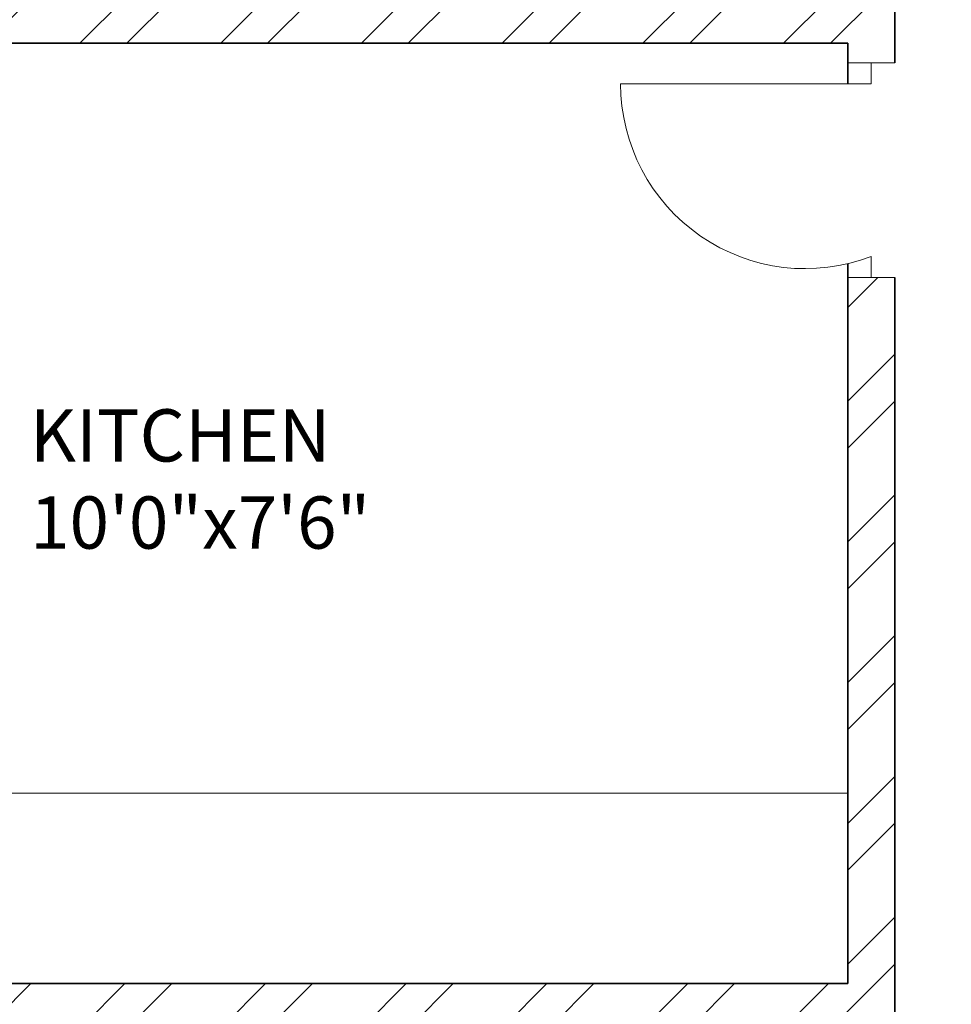
# Model space of a CAD drawing. Units: inches. Extents: x 1885 to 2748, y 783 to 2421.
# Tile 79 of 117: x 2038 to 2127, y 2073 to 2167. Entities that reach past the tile are written whole.
import ezdxf

# ---------------------------------------------------------------- set-up
doc = ezdxf.new("R2010")
doc.units = ezdxf.units.IN
for name, color, linetype, lineweight in [('A-AREA-IDEN', 7, 'Continuous', 18), ('A-DOOR', 31, 'Continuous', 18), ('A-FLOR-CASE', 9, 'Continuous', 18), ('A-WALL', 7, 'Continuous', 35)]:
    doc.layers.add(name, color=color, linetype=linetype, lineweight=lineweight)
doc.layers.add('A-WALL-PATT', color=85, linetype='Continuous', lineweight=13, true_color=0x58ba48)
doc.styles.get("Standard").update_dxf_attribs({"font": 'arial.ttf'})

msp = doc.modelspace()

# ---------------------------------------------------------------- hatches: boundary and pattern name
at = {"layer": 'A-WALL-PATT'}
h = msp.add_hatch(dxfattribs=at)
h.set_pattern_fill('ANSI32', color=256)
h.paths.add_polyline_path([(2007.772, 2318.006), (1980.774, 2318.006), (1980.774, 2281.215), (1985.274, 2281.215), (1985.274, 2313.506), (2007.772, 2313.506), (2007.772, 2315.756)])
h.paths.add_polyline_path([(2094.324, 2318.006), (2067.772, 2318.006), (2067.772, 2313.506), (2094.324, 2313.506), (2094.324, 2315.756)])
h.paths.add_polyline_path([(2131.367, 2315.756), (2131.367, 2318.006), (2131.189, 2318.006), (2112.609, 2318.006), (2112.609, 2313.506), (2117.274, 2313.506), (2117.274, 2255.201), (2121.774, 2255.201), (2121.774, 2313.506), (2131.367, 2313.506)])
h.paths.add_polyline_path([(2190.512, 2318.006), (2155.367, 2318.006), (2155.367, 2313.506), (2169.774, 2313.506), (2169.774, 2229.506), (2121.774, 2229.506), (2121.774, 2233.451), (2119.524, 2233.451), (2117.274, 2233.451), (2117.274, 2201.101), (2121.774, 2201.101), (2121.774, 2225.006), (2169.774, 2225.006), (2169.774, 2165.006), (2306.274, 2165.006), (2306.274, 2066.006), (2310.774, 2066.006), (2344.274, 2066.006), (2486.274, 2066.006), (2486.274, 1886.006), (2483.02, 1886.006), (2483.02, 1881.506), (2486.274, 1881.506), (2486.274, 1880.678), (2490.774, 1880.678), (2490.774, 2070.506), (2344.274, 2070.506), (2310.774, 2070.506), (2310.774, 2165.006), (2310.774, 2173.636), (2308.524, 2173.636), (2306.274, 2173.636), (2306.274, 2169.506), (2174.274, 2169.506), (2174.274, 2313.506), (2190.512, 2313.506), (2190.512, 2315.756)])
h.paths.add_polyline_path([(1985.274, 2221.215), (1980.774, 2221.215), (1980.774, 2165.006), (1992.774, 2165.006), (1992.774, 2141.927), (1997.274, 2141.927), (1997.274, 2165.006), (2117.274, 2165.006), (2117.274, 2163.126), (2121.774, 2163.126), (2121.774, 2172.734), (2119.524, 2172.734), (2117.274, 2172.734), (2117.274, 2169.506), (1985.274, 2169.506)])
h.paths.add_polyline_path([(1997.274, 2105.927), (1992.774, 2105.927), (1992.774, 2070.506), (2016.774, 2070.506), (2016.774, 2059.123), (2019.024, 2059.123), (2021.274, 2059.123), (2021.274, 2070.506), (2117.274, 2070.506), (2117.274, 2022.506), (2114.423, 2022.506), (2114.423, 2018.006), (2123.627, 2018.006), (2123.627, 2020.256), (2123.627, 2022.506), (2121.774, 2022.506), (2121.774, 2142.587), (2119.524, 2142.587), (2117.274, 2142.587), (2117.274, 2075.006), (1997.274, 2075.006)])
h.paths.add_polyline_path([(2092.029, 2020.256), (2092.029, 2022.506), (2021.274, 2022.506), (2021.274, 2035.123), (2016.774, 2035.123), (2016.774, 2018.006), (2016.774, 1978.784), (2021.274, 1978.784), (2021.274, 2018.006), (2092.029, 2018.006)])
h.paths.add_polyline_path([(2260.938, 2022.506), (2153.105, 2022.506), (2153.105, 2020.256), (2153.105, 2018.006), (2155.274, 2018.006), (2155.274, 1886.006), (2107.629, 1886.006), (2107.629, 1881.506), (2182.911, 1881.506), (2182.911, 1883.756), (2182.911, 1886.006), (2159.774, 1886.006), (2159.774, 2018.006), (2260.938, 2018.006), (2260.938, 2020.256)])
h.paths.add_polyline_path([(2047.629, 1883.756), (2047.629, 1886.006), (2021.274, 1886.006), (2021.274, 1918.784), (2019.024, 1918.784), (2016.774, 1918.784), (2016.774, 1881.506), (2047.629, 1881.506)])
h.paths.add_polyline_path([(2306.361, 1883.756), (2306.361, 1886.006), (2296.274, 1886.006), (2296.274, 1982.006), (2316.535, 1982.006), (2316.535, 1984.256), (2316.535, 1986.506), (2296.274, 1986.506), (2296.274, 2022.506), (2289.276, 2022.506), (2289.276, 2018.006), (2291.774, 2018.006), (2291.774, 1886.006), (2242.911, 1886.006), (2242.911, 1881.506), (2306.361, 1881.506)], flags=17)
h.paths.add_polyline_path([(1985.274, 1843.006), (2021.6, 1843.006), (2021.534, 1845.441), (2021.477, 1847.506), (1980.774, 1847.506), (1980.774, 1809.446), (1985.274, 1809.446)])
h.paths.add_polyline_path([(2131.482, 1845.256), (2131.482, 1847.506), (2081.534, 1847.506), (2081.534, 1843.006), (2117.274, 1843.006), (2117.274, 1784.147), (2119.524, 1784.147), (2121.774, 1784.147), (2121.774, 1843.006), (2131.482, 1843.006)])
h.paths.add_polyline_path([(2203.886, 1847.506), (2155.482, 1847.506), (2155.482, 1843.006), (2169.774, 1843.006), (2169.774, 1759.006), (2121.774, 1759.006), (2121.774, 1761.457), (2117.274, 1761.457), (2117.274, 1730.429), (2121.774, 1730.429), (2121.774, 1754.506), (2177.421, 1754.506), (2177.421, 1756.756), (2177.421, 1759.006), (2174.274, 1759.006), (2174.274, 1843.006), (2203.886, 1843.006)])
h.paths.add_polyline_path([(2335.554, 1845.256), (2335.554, 1847.506), (2239.886, 1847.506), (2239.886, 1843.006), (2306.274, 1843.006), (2306.274, 1759.006), (2199.486, 1759.006), (2199.486, 1754.506), (2310.774, 1754.506), (2310.774, 1843.006), (2335.554, 1843.006)])
h.paths.add_polyline_path([(2348.774, 2022.506), (2344.274, 2022.506), (2344.274, 1986.506), (2341.681, 1986.506), (2341.681, 1982.006), (2344.274, 1982.006), (2344.274, 1886.006), (2330.361, 1886.006), (2330.361, 1881.506), (2361.627, 1881.506), (2361.627, 1883.756), (2361.627, 1886.006), (2348.774, 1886.006)], flags=17)
h.paths.add_polyline_path([(2283.251, 2315.756), (2283.251, 2318.006), (2238.512, 2318.006), (2238.512, 2313.506), (2283.251, 2313.506)], flags=17)
h.paths.add_polyline_path([(2363.274, 2348.006), (2388.677, 2348.006), (2388.677, 2350.256), (2388.677, 2352.506), (2358.774, 2352.506), (2358.774, 2348.006), (2358.774, 2318.006), (2344.481, 2318.006), (2344.481, 2313.506), (2358.774, 2313.506), (2358.774, 2229.506), (2310.774, 2229.506), (2310.774, 2231.952), (2306.274, 2231.952), (2306.274, 2205.611), (2310.774, 2205.611), (2310.774, 2225.006), (2358.774, 2225.006), (2358.774, 2211.506), (2452.329, 2211.506), (2452.329, 2213.756), (2452.329, 2216.006), (2363.274, 2216.006), (2363.274, 2318.006)])
h.paths.add_polyline_path([(2310.774, 2313.506), (2320.481, 2313.506), (2320.481, 2315.756), (2320.481, 2318.006), (2302.728, 2318.006), (2302.728, 2313.506), (2306.274, 2313.506), (2306.274, 2251.076), (2310.774, 2251.076)], flags=17)
h.paths.add_polyline_path([(2490.774, 2352.506), (2486.274, 2352.506), (2448.677, 2352.506), (2448.677, 2348.006), (2486.274, 2348.006), (2486.274, 2318.006), (2486.274, 2216.006), (2481.78, 2216.006), (2481.78, 2211.506), (2486.274, 2211.506), (2486.274, 2165.006), (2493.289, 2165.006), (2493.289, 2167.256), (2493.289, 2169.506), (2490.774, 2169.506), (2490.774, 2313.506), (2494.429, 2313.506), (2494.429, 2318.006), (2490.774, 2318.006)])
h.paths.add_polyline_path([(2534.653, 2318.006), (2515.691, 2318.006), (2515.691, 2313.506), (2534.653, 2313.506), (2534.653, 2315.756)])
h.paths.add_polyline_path([(2618.274, 2318.006), (2594.653, 2318.006), (2594.653, 2313.506), (2613.774, 2313.506), (2613.774, 2281.706), (2618.274, 2281.706)])
h.paths.add_polyline_path([(2618.274, 2221.706), (2613.774, 2221.706), (2613.774, 2169.506), (2554.019, 2169.506), (2554.019, 2165.006), (2613.774, 2165.006), (2613.774, 2152.878), (2618.274, 2152.878)])
h.paths.add_polyline_path([(2618.274, 2128.878), (2616.024, 2128.878), (2613.774, 2128.878), (2613.774, 2117.006), (2529.774, 2117.006), (2529.774, 2165.006), (2532.848, 2165.006), (2532.848, 2169.506), (2522.867, 2169.506), (2522.867, 2165.006), (2525.274, 2165.006), (2525.274, 2117.006), (2525.274, 2112.506), (2525.274, 2108.576), (2529.774, 2108.576), (2529.774, 2112.506), (2613.774, 2112.506), (2613.774, 2080.19), (2618.274, 2080.19)])
h.paths.add_polyline_path([(2618.274, 2044.19), (2616.024, 2044.19), (2613.774, 2044.19), (2613.774, 2015.506), (2529.774, 2015.506), (2529.774, 2088.582), (2527.524, 2088.582), (2525.274, 2088.582), (2525.274, 2011.006), (2613.774, 2011.006), (2613.774, 1956.755), (2618.274, 1956.755)])
h.paths.add_polyline_path([(2618.274, 1881.506), (2618.274, 1896.755), (2613.774, 1896.755), (2613.774, 1881.506), (2613.774, 1847.506), (2592.715, 1847.506), (2592.715, 1843.006), (2613.774, 1843.006), (2613.774, 1765.006), (2613.774, 1760.506), (2609.621, 1760.506), (2609.621, 1756.006), (2613.774, 1756.006), (2613.774, 1660.006), (2608.544, 1660.006), (2608.544, 1655.506), (2613.774, 1655.506), (2613.774, 1508.158), (2618.274, 1508.158)])
h.paths.add_polyline_path([(2565.774, 1843.006), (2568.997, 1843.006), (2568.997, 1847.506), (2490.774, 1847.506), (2490.774, 1849.7), (2488.524, 1849.7), (2486.274, 1849.7), (2486.274, 1847.506), (2477.274, 1847.506), (2477.274, 1838.506), (2477.274, 1821.493), (2486.274, 1821.493), (2486.274, 1838.506), (2561.274, 1838.506), (2561.274, 1765.006), (2486.274, 1765.006), (2486.274, 1786.157), (2477.274, 1786.157), (2477.274, 1765.006), (2477.274, 1756.006), (2486.274, 1756.006), (2565.774, 1756.006), (2585.621, 1756.006), (2585.621, 1758.256), (2585.621, 1760.506), (2565.774, 1760.506), (2565.774, 1765.006)])
h.paths.add_polyline_path([(2486.274, 1651.006), (2561.274, 1651.006), (2561.274, 1567.006), (2486.274, 1567.006), (2486.274, 1591.321), (2477.274, 1591.321), (2477.274, 1567.006), (2477.274, 1558.006), (2477.274, 1555.439), (2481.774, 1555.439), (2481.774, 1558.006), (2568.653, 1558.006), (2568.653, 1560.256), (2568.653, 1562.506), (2565.774, 1562.506), (2565.774, 1655.506), (2584.544, 1655.506), (2584.544, 1657.756), (2584.544, 1660.006), (2565.774, 1660.006), (2486.274, 1660.006), (2477.274, 1660.006), (2477.274, 1651.006), (2477.274, 1632.989), (2486.274, 1632.989)])
h.paths.add_polyline_path([(2449.967, 1883.756), (2449.967, 1886.006), (2421.627, 1886.006), (2421.627, 1881.506), (2449.967, 1881.506)], flags=17)
h.paths.add_polyline_path([(2447.274, 1847.506), (2395.554, 1847.506), (2395.554, 1843.006), (2442.774, 1843.006), (2442.774, 1809.27), (2447.274, 1809.27)])
h.paths.add_polyline_path([(1985.274, 1749.446), (1980.774, 1749.446), (1980.774, 1694.504), (1985.274, 1694.504), (1985.274, 1694.506), (1986.897, 1694.506), (1986.897, 1697.78), (1986.897, 1699.006), (1985.274, 1699.006)])
h.paths.add_polyline_path([(2152.774, 1699.006), (2121.774, 1699.006), (2121.774, 1703.668), (2119.524, 1703.668), (2117.274, 1703.668), (2117.274, 1699.006), (2009.219, 1699.006), (2009.219, 1694.506), (2148.274, 1694.506), (2148.274, 1692.631), (2152.774, 1692.631)])
h.paths.add_polyline_path([(2016.274, 1694.506), (2011.774, 1694.506), (2011.774, 1558.006), (2040.806, 1558.006), (2040.806, 1560.256), (2040.806, 1562.506), (2016.274, 1562.506)])
h.paths.add_polyline_path([(2152.774, 1663.017), (2150.524, 1663.017), (2148.274, 1663.017), (2148.274, 1562.506), (2100.806, 1562.506), (2100.806, 1558.006), (2165.119, 1558.006), (2165.119, 1560.256), (2165.119, 1562.506), (2152.774, 1562.506), (2152.774, 1610.506), (2224.774, 1610.506), (2224.774, 1607.99), (2229.274, 1607.99), (2229.274, 1615.006), (2152.774, 1615.006)])
h.paths.add_polyline_path([(2238.613, 1560.256), (2238.613, 1562.506), (2229.274, 1562.506), (2229.274, 1588.756), (2227.024, 1588.763), (2224.774, 1588.771), (2224.774, 1562.506), (2189.119, 1562.506), (2189.119, 1558.006), (2238.613, 1558.006)])
h.paths.add_polyline_path([(2336.024, 1560.256), (2336.024, 1562.506), (2310.774, 1562.506), (2310.774, 1656.347), (2308.524, 1656.347), (2306.274, 1656.347), (2306.274, 1562.506), (2286.613, 1562.506), (2286.613, 1558.006), (2336.024, 1558.006)])
h.paths.add_polyline_path([(2447.274, 1690.968), (2445.024, 1690.968), (2442.774, 1690.968), (2442.774, 1687.006), (2306.274, 1687.006), (2306.274, 1680.75), (2310.774, 1680.75), (2310.774, 1682.506), (2442.774, 1682.506), (2442.774, 1562.506), (2396.024, 1562.506), (2396.024, 1558.006), (2447.274, 1558.006)])
h.paths.add_polyline_path([(2447.274, 1749.27), (2445.024, 1749.27), (2442.774, 1749.27), (2442.774, 1717.232), (2447.274, 1717.232)])
h.paths.add_polyline_path([(2044.674, 1521.756), (2044.674, 1524.006), (2007.274, 1524.006), (2007.274, 1503.49), (2009.524, 1503.49), (2011.774, 1503.49), (2011.774, 1519.506), (2044.674, 1519.506)])
h.paths.add_polyline_path([(2177.969, 1521.756), (2177.969, 1524.006), (2104.674, 1524.006), (2104.674, 1519.506), (2145.774, 1519.506), (2145.774, 1387.506), (2143.37, 1387.506), (2143.37, 1383.006), (2251.585, 1383.006), (2251.585, 1385.256), (2251.585, 1387.506), (2150.274, 1387.506), (2150.274, 1519.506), (2177.969, 1519.506)])
h.paths.add_polyline_path([(2298.704, 1524.006), (2237.969, 1524.006), (2237.969, 1519.506), (2282.274, 1519.506), (2282.274, 1387.506), (2279.683, 1387.506), (2279.683, 1383.006), (2286.774, 1383.006), (2286.774, 1419.006), (2312.451, 1419.006), (2312.451, 1421.256), (2312.451, 1423.506), (2286.774, 1423.506), (2286.774, 1519.506), (2298.704, 1519.506), (2298.704, 1521.722)], flags=17)
h.paths.add_polyline_path([(2361.897, 1521.756), (2361.897, 1524.006), (2322.704, 1524.006), (2322.704, 1519.506), (2334.774, 1519.506), (2334.774, 1423.506), (2331.93, 1423.506), (2331.93, 1419.006), (2334.774, 1419.006), (2334.774, 1387.506), (2334.774, 1383.228), (2339.274, 1383.228), (2339.274, 1387.506), (2339.274, 1519.506), (2361.897, 1519.506)], flags=17)
h.paths.add_polyline_path([(2447.274, 1521.756), (2447.274, 1524.006), (2421.897, 1524.006), (2421.897, 1519.506), (2447.274, 1519.506)], flags=17)
h.paths.add_polyline_path([(2481.774, 1529.6), (2479.524, 1529.6), (2477.274, 1529.6), (2477.274, 1524.006), (2474.489, 1524.006), (2474.489, 1519.506), (2477.274, 1519.506), (2477.274, 1334.506), (2296.774, 1334.506), (2296.774, 1240.506), (2160.274, 1240.506), (2160.274, 1180.506), (2112.274, 1180.506), (2112.274, 1207.692), (2110.024, 1207.692), (2107.774, 1207.692), (2107.774, 1171.609), (2112.274, 1171.609), (2112.274, 1176.006), (2160.274, 1176.006), (2160.274, 1092.006), (2144.221, 1092.006), (2144.221, 1087.506), (2189.497, 1087.506), (2189.497, 1089.756), (2189.497, 1092.006), (2164.774, 1092.006), (2164.774, 1236.006), (2296.774, 1236.006), (2296.774, 1231.912), (2301.274, 1231.912), (2301.274, 1330.006), (2481.774, 1330.006), (2481.774, 1387.506)])
h.paths.add_polyline_path([(2618.274, 1448.158), (2613.774, 1448.158), (2613.774, 1382.506), (2529.774, 1382.506), (2525.274, 1382.506), (2525.274, 1307.062), (2529.774, 1307.062), (2529.774, 1378.006), (2613.774, 1378.006), (2613.774, 1354.988), (2618.274, 1354.988)])
h.paths.add_polyline_path([(2618.274, 1318.988), (2613.774, 1318.988), (2613.774, 1281.006), (2529.774, 1281.006), (2529.774, 1283.786), (2527.524, 1283.786), (2525.274, 1283.786), (2525.274, 1228.506), (2516.794, 1228.506), (2516.794, 1224.006), (2533.484, 1224.006), (2533.484, 1226.256), (2533.484, 1228.506), (2529.774, 1228.506), (2529.774, 1276.506), (2613.774, 1276.506), (2613.774, 1266.02), (2618.274, 1266.02)])
h.paths.add_polyline_path([(2618.274, 1134.964), (2613.774, 1134.964), (2613.774, 1092.006), (2594.545, 1092.006), (2594.545, 1087.506), (2618.274, 1087.506)])
h.paths.add_polyline_path([(2534.545, 1092.006), (2509.765, 1092.006), (2509.765, 1087.506), (2534.545, 1087.506), (2534.545, 1089.756)])
h.paths.add_polyline_path([(2481.274, 1224.006), (2484.117, 1224.006), (2484.117, 1226.256), (2484.117, 1228.506), (2476.774, 1228.506), (2476.774, 1198.506), (2471.61, 1198.506), (2471.61, 1194.006), (2476.774, 1194.006), (2476.774, 1062.006), (2436.894, 1062.006), (2436.894, 1057.506), (2476.774, 1057.506), (2481.274, 1057.506), (2481.274, 1062.006), (2481.274, 1087.506), (2485.354, 1087.506), (2485.354, 1089.756), (2485.354, 1092.006), (2481.274, 1092.006), (2481.274, 1117.506)])
h.paths.add_polyline_path([(2439.898, 1198.506), (2349.274, 1198.506), (2349.274, 1194.006), (2349.274, 1180.506), (2301.274, 1180.506), (2301.274, 1201.896), (2299.024, 1201.896), (2296.774, 1201.896), (2296.774, 1172.335), (2299.024, 1172.335), (2301.274, 1172.335), (2301.274, 1176.006), (2349.274, 1176.006), (2349.274, 1092.006), (2334.452, 1092.006), (2334.452, 1087.506), (2349.274, 1087.506), (2349.274, 1057.506), (2353.774, 1057.506), (2376.894, 1057.506), (2376.894, 1059.756), (2376.894, 1062.006), (2353.774, 1062.006), (2353.774, 1087.506), (2353.774, 1180.506), (2353.774, 1194.006), (2439.898, 1194.006), (2439.898, 1196.256)])
h.paths.add_polyline_path([(2270.596, 1089.756), (2270.596, 1092.006), (2249.497, 1092.006), (2249.497, 1087.506), (2270.596, 1087.506)], flags=17)
h.paths.add_polyline_path([(2310.452, 1092.006), (2301.274, 1092.006), (2301.274, 1153.292), (2296.774, 1153.292), (2296.774, 1092.006), (2293.786, 1092.006), (2293.786, 1087.506), (2310.452, 1087.506), (2310.452, 1089.756)], flags=17)
h.paths.add_polyline_path([(2112.274, 1150.328), (2110.024, 1150.328), (2107.774, 1150.328), (2107.774, 1092.006), (2104.465, 1092.006), (2104.465, 1087.506), (2120.221, 1087.506), (2120.221, 1089.756), (2120.221, 1092.006), (2112.274, 1092.006)])
h.paths.add_polyline_path([(2082.172, 1092.006), (2058.144, 1092.006), (2058.144, 1087.506), (2082.172, 1087.506), (2082.172, 1089.756)])
h.paths.add_polyline_path([(1975.774, 1145.638), (1971.274, 1145.638), (1971.274, 1087.506), (1980.774, 1087.506), (1998.144, 1087.506), (1998.144, 1089.756), (1998.144, 1092.006), (1985.274, 1092.006), (1975.774, 1092.006)])
h.paths.add_polyline_path([(2112.274, 1244.385), (2110.024, 1244.385), (2107.774, 1244.385), (2107.774, 1240.506), (1992.274, 1240.506), (1992.274, 1271.008), (1987.774, 1271.008), (1987.774, 1240.506), (1980.774, 1240.506), (1975.774, 1240.506), (1971.274, 1240.506), (1971.274, 1205.638), (1975.774, 1205.638), (1975.774, 1236.006), (2107.774, 1236.006), (2107.774, 1233.444), (2112.274, 1233.444), (2112.274, 1236.006)])
h.paths.add_polyline_path([(2112.274, 1383.006), (2114.783, 1383.006), (2114.783, 1385.256), (2114.783, 1387.506), (2102.476, 1387.506), (2102.476, 1383.006), (2107.774, 1383.006), (2107.774, 1335.006), (2011.774, 1335.006), (2011.774, 1349.939), (2007.274, 1349.939), (2007.274, 1335.006), (1987.774, 1335.006), (1987.774, 1330.506), (1987.774, 1307.008), (1992.274, 1307.008), (1992.274, 1330.506), (2007.274, 1330.506), (2107.774, 1330.506), (2107.774, 1264.711), (2112.274, 1264.711)])
h.paths.add_polyline_path([(2077.857, 1387.506), (2011.774, 1387.506), (2011.774, 1390.036), (2009.524, 1390.036), (2007.274, 1390.036), (2007.274, 1373.939), (2011.774, 1373.939), (2011.774, 1383.006), (2077.857, 1383.006)])
h.paths.add_polyline_path([(2011.774, 1443.49), (2007.274, 1443.49), (2007.274, 1410.248), (2011.774, 1410.248)])

# ---------------------------------------------------------------- linework, layer by layer
at = {"layer": 'A-DOOR'}
for p, q in [((2117.274, 2163.126), (2121.774, 2163.126)), ((2121.774, 2163.126), (2119.524, 2163.126)), ((2119.524, 2163.126), (2119.524, 2161.126)), ((2119.524, 2161.126), (2095.524, 2161.126)), ((2119.524, 2142.587), (2119.524, 2144.587)), ((2117.274, 2142.587), (2121.774, 2142.587)), ((2121.774, 2142.587), (2119.524, 2142.587))]:
    msp.add_line(p, q, dxfattribs=at)
msp.add_arc((2113.223, 2161.126), 17.699, 180, 290.85509, dxfattribs=at)
at = {"layer": 'A-FLOR-CASE'}
msp.add_line((2013.676, 2093.221), (2117.274, 2093.221), dxfattribs=at)
at = {"layer": 'A-WALL'}
for p, q in [((2121.774, 2172.734), (2121.774, 2163.126)), ((1997.274, 2165.006), (2117.274, 2165.006)), ((2117.274, 2165.006), (2117.274, 2161.126)), ((2117.274, 2143.897), (2117.274, 2075.006)), ((2121.774, 2142.587), (2121.774, 2022.506)), ((1997.274, 2075.006), (2117.274, 2075.006))]:
    msp.add_line(p, q, dxfattribs=at)

# ---------------------------------------------------------------- texts
at = {"layer": 'A-AREA-IDEN', "insert": (2038.987, 2129.965), "char_height": 5, "attachment_point": 1}
msp.add_mtext_dynamic_manual_height_columns('KITCHEN\\P10\'0"x7\'6"', width=112.94094, gutter_width=12.5, heights=[0], dxfattribs=at)

doc.saveas('drawing.dxf')
